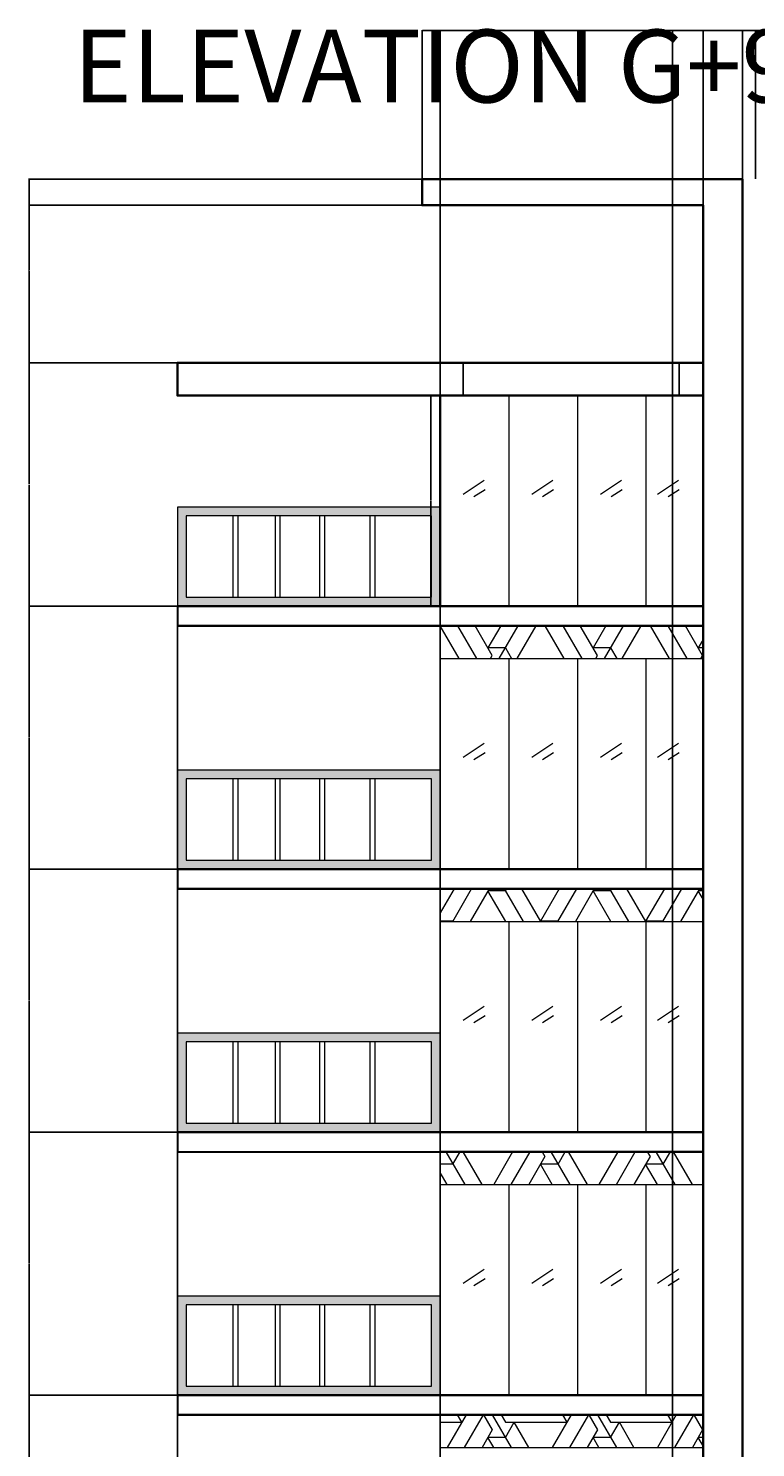
# Model space of a CAD drawing. Units: inches. Extents: x -38 to 698, y -57 to 1364.
# Tile 4 of 5: x -38 to 294, y 716 to 1364. Entities that reach past the tile are written whole.
import ezdxf

# ---------------------------------------------------------------- set-up
doc = ezdxf.new("R2010")
doc.units = ezdxf.units.IN
doc.header["$MEASUREMENT"] = 0
for name, color, linetype, lineweight in [('A-ANNO-DIMS', 2, 'Continuous', 18), ('A-ANNO-TEXT', 7, 'Continuous', 25), ('A-ELEV-PATT', 8, 'Continuous', 13), ('A-FLOR', 7, 'Continuous', 30), ('A-FLOR-HRAL', 7, 'Continuous', 20), ('A-GLAZ', 4, 'Continuous', 18), ('A-ROOF', 7, 'Continuous', 35), ('A-WALL', 7, 'Continuous', 35), ('A-WALL-PATT', 8, 'Continuous', 13)]:
    doc.layers.add(name, color=color, linetype=linetype, lineweight=lineweight)
doc.styles.get("Standard").update_dxf_attribs({"font": 'arial.ttf'})
doc.dimstyles.get("Standard").update_dxf_attribs({"dimtxt": 0.18, "dimasz": 0.18, "dimexe": 0.18, "dimexo": 0.0625, "dimgap": 0.09, "dimtad": 0, "dimtih": 1, "dimtoh": 1, "dimdec": 4, "dimzin": 0, "dimdsep": 46, "dimtxsty": 'Standard', "dimcen": 0.09, "dimadec": 0, "dimazin": 0, "dimtfac": 1, "dimtdec": 4, "dimtofl": 0, "dimtmove": 0, "dimatfit": 3, "dimfxl": 1, "dimtolj": 1, "dimtzin": 0, "dimarcsym": 0})

# ---------------------------------------------------------------- blocks, each defined once
blk = doc.blocks.new('WINDOW-4L-LH')
for p, q in [((20.81, 96), (20.81, 0)), ((52.11, 96), (52.11, 0)), ((83.42, 96), (83.42, 0)), ((0, 50.99), (9.6, 57.46)), ((4.92, 50.03), (9.96, 53.14)), ((31.3, 50.99), (40.9, 57.46)), ((36.22, 50.03), (41.26, 53.14)), ((62.61, 50.99), (72.2, 57.46)), ((67.52, 50.03), (72.56, 53.14)), ((88.7, 50.99), (98.29, 57.46)), ((93.61, 50.03), (98.65, 53.14))]:
    blk.add_line(p, q)
blk = doc.blocks.new('BALCONY-GUARD-PICKETS')
for p, q in [((0, 37.13), (0, 0)), ((2.41, 0), (2.41, 37.13)), ((19.25, 37.13), (19.25, 0)), ((21.65, 0), (21.65, 37.13)), ((39.53, 37.13), (39.53, 0)), ((41.93, 0), (41.93, 37.13)), ((62.55, 37.13), (62.55, 0)), ((64.96, 0), (64.96, 37.13))]:
    blk.add_line(p, q)
blk = doc.blocks.new('*D10')
at = {"layer": 'A-ANNO-DIMS', "color": 0, "lineweight": -2, "transparency": 16777216}
for p, q in [((160.18, 1196.28), (160.18, 1211.19)), ((160.36, 1211.01), (208.2, 1211.01)), ((258.65, 1211.01), (210.81, 1211.01)), ((258.83, 1196.28), (258.83, 1211.19))]:
    blk.add_line(p, q, dxfattribs=at)
at = {"layer": 'A-ANNO-DIMS', "color": 0, "transparency": 16777216}
for points in [[(160.36, 1211.04), (160.36, 1210.98), (160.18, 1211.01)], [(258.65, 1211.04), (258.65, 1210.98), (258.83, 1211.01)]]:
    blk.add_solid(points, dxfattribs=at)
at = {"layer": 'Defpoints', "color": 0, "transparency": 16777216}
for p in [(258.83, 1211.01), (160.18, 1196.21), (258.83, 1196.21)]:
    blk.add_point(p, dxfattribs=at)
at = {"layer": 'A-ANNO-DIMS', "color": 0, "transparency": 16777216, "insert": (209.51, 1211.01), "char_height": 0.18, "attachment_point": 5}
blk.add_mtext('\\A1;LH WINDOW 99 TYP.', dxfattribs=at)
blk = doc.blocks.new('*D11')
at = {"layer": 'A-ANNO-DIMS', "color": 0, "lineweight": -2, "transparency": 16777216}
for p, q in [((160.12, 1196.21), (145.2, 1196.21)), ((145.38, 1196.03), (145.38, 1148.4)), ((145.38, 1100.39), (145.38, 1148.03)), ((160.12, 1100.21), (145.2, 1100.21))]:
    blk.add_line(p, q, dxfattribs=at)
at = {"layer": 'A-ANNO-DIMS', "color": 0, "transparency": 16777216}
for points in [[(145.35, 1196.03), (145.41, 1196.03), (145.38, 1196.21)], [(145.35, 1100.39), (145.41, 1100.39), (145.38, 1100.21)]]:
    blk.add_solid(points, dxfattribs=at)
at = {"layer": 'Defpoints', "color": 0, "transparency": 16777216}
for p in [(145.38, 1196.21), (160.18, 1196.21), (160.18, 1100.21)]:
    blk.add_point(p, dxfattribs=at)
at = {"layer": 'A-ANNO-DIMS', "color": 0, "transparency": 16777216, "insert": (145.38, 1148.21), "char_height": 0.18, "attachment_point": 5}
blk.add_mtext('\\A1;96 TYP.', dxfattribs=at)
blk = doc.blocks.new('*D24')
at = {"layer": 'A-ANNO-DIMS', "color": 0, "lineweight": -2, "transparency": 16777216}
for p, q in [((29.69, 1100.15), (29.69, -56.67)), ((269.69, 1100.15), (269.69, -56.67)), ((29.87, -56.49), (149.4, -56.49)), ((269.51, -56.49), (149.98, -56.49))]:
    blk.add_line(p, q, dxfattribs=at)
at = {"layer": 'A-ANNO-DIMS', "color": 0, "transparency": 16777216}
for points in [[(29.87, -56.46), (29.87, -56.52), (29.69, -56.49)], [(269.51, -56.46), (269.51, -56.52), (269.69, -56.49)]]:
    blk.add_solid(points, dxfattribs=at)
at = {"layer": 'Defpoints', "color": 0, "transparency": 16777216}
for p in [(29.69, 1100.21), (269.69, 1100.21), (269.69, -56.49)]:
    blk.add_point(p, dxfattribs=at)
at = {"layer": 'A-ANNO-DIMS', "color": 0, "transparency": 16777216, "insert": (149.69, -56.49), "char_height": 0.18, "attachment_point": 5}
blk.add_mtext('\\A1;240', dxfattribs=at)
blk = doc.blocks.new('*D25')
at = {"layer": 'A-ANNO-DIMS', "color": 0, "lineweight": -2, "transparency": 16777216}
for p, q in [((269.69, 1100.15), (269.69, -56.67)), ((389.69, 1100.15), (389.69, -56.67)), ((269.87, -56.49), (329.41, -56.49)), ((389.51, -56.49), (329.97, -56.49))]:
    blk.add_line(p, q, dxfattribs=at)
at = {"layer": 'A-ANNO-DIMS', "color": 0, "transparency": 16777216}
for points in [[(269.87, -56.46), (269.87, -56.52), (269.69, -56.49)], [(389.51, -56.46), (389.51, -56.52), (389.69, -56.49)]]:
    blk.add_solid(points, dxfattribs=at)
at = {"layer": 'Defpoints', "color": 0, "transparency": 16777216}
for p in [(269.69, 1100.21), (389.69, 1100.21), (389.69, -56.49)]:
    blk.add_point(p, dxfattribs=at)
at = {"layer": 'A-ANNO-DIMS', "color": 0, "transparency": 16777216, "insert": (329.69, -56.49), "char_height": 0.18, "attachment_point": 5}
blk.add_mtext('\\A1;120', dxfattribs=at)
blk = doc.blocks.new('*D27')
at = {"layer": 'A-ANNO-DIMS', "color": 0, "lineweight": -2, "transparency": 16777216}
for p, q in [((149.69, 380.28), (149.69, 1362.92)), ((149.87, 1362.74), (209.41, 1362.74)), ((269.51, 1362.74), (209.97, 1362.74)), ((269.69, 380.28), (269.69, 1362.92))]:
    blk.add_line(p, q, dxfattribs=at)
at = {"layer": 'A-ANNO-DIMS', "color": 0, "transparency": 16777216}
for points in [[(149.87, 1362.77), (149.87, 1362.71), (149.69, 1362.74)], [(269.51, 1362.77), (269.51, 1362.71), (269.69, 1362.74)]]:
    blk.add_solid(points, dxfattribs=at)
at = {"layer": 'Defpoints', "color": 0, "transparency": 16777216}
for p in [(269.69, 1362.74), (149.69, 380.21), (269.69, 380.21)]:
    blk.add_point(p, dxfattribs=at)
at = {"layer": 'A-ANNO-DIMS', "color": 0, "transparency": 16777216, "insert": (209.69, 1362.74), "char_height": 0.18, "attachment_point": 5}
blk.add_mtext('\\A1;120', dxfattribs=at)
blk = doc.blocks.new('*D34')
at = {"layer": 'A-ANNO-DIMS', "color": 0, "lineweight": -2, "transparency": 16777216}
for p, q in [((29.62, 740.21), (-38.19, 740.21)), ((-38.01, 740.03), (-38.01, 680.4)), ((-38.01, 620.39), (-38.01, 680.03)), ((29.62, 620.21), (-38.19, 620.21))]:
    blk.add_line(p, q, dxfattribs=at)
at = {"layer": 'A-ANNO-DIMS', "color": 0, "transparency": 16777216}
for points in [[(-38.04, 740.03), (-37.98, 740.03), (-38.01, 740.21)], [(-38.04, 620.39), (-37.98, 620.39), (-38.01, 620.21)]]:
    blk.add_solid(points, dxfattribs=at)
at = {"layer": 'Defpoints', "color": 0, "transparency": 16777216}
for p in [(-38.01, 740.21), (29.69, 740.21), (29.69, 620.21)]:
    blk.add_point(p, dxfattribs=at)
at = {"layer": 'A-ANNO-DIMS', "color": 0, "transparency": 16777216, "insert": (-38.01, 680.21), "char_height": 0.18, "attachment_point": 5}
blk.add_mtext('\\A1;120', dxfattribs=at)
blk = doc.blocks.new('*D35')
at = {"layer": 'A-ANNO-DIMS', "color": 0, "lineweight": -2, "transparency": 16777216}
for p, q in [((29.62, 860.21), (-38.19, 860.21)), ((-38.01, 860.03), (-38.01, 800.4)), ((-38.01, 740.39), (-38.01, 800.03)), ((29.62, 740.21), (-38.19, 740.21))]:
    blk.add_line(p, q, dxfattribs=at)
at = {"layer": 'A-ANNO-DIMS', "color": 0, "transparency": 16777216}
for points in [[(-38.04, 860.03), (-37.98, 860.03), (-38.01, 860.21)], [(-38.04, 740.39), (-37.98, 740.39), (-38.01, 740.21)]]:
    blk.add_solid(points, dxfattribs=at)
at = {"layer": 'Defpoints', "color": 0, "transparency": 16777216}
for p in [(-38.01, 860.21), (29.69, 860.21), (29.69, 740.21)]:
    blk.add_point(p, dxfattribs=at)
at = {"layer": 'A-ANNO-DIMS', "color": 0, "transparency": 16777216, "insert": (-38.01, 800.21), "char_height": 0.18, "attachment_point": 5}
blk.add_mtext('\\A1;120', dxfattribs=at)
blk = doc.blocks.new('*D36')
at = {"layer": 'A-ANNO-DIMS', "color": 0, "lineweight": -2, "transparency": 16777216}
for p, q in [((29.62, 980.21), (-38.19, 980.21)), ((-38.01, 980.03), (-38.01, 920.4)), ((-38.01, 860.39), (-38.01, 920.03)), ((29.62, 860.21), (-38.19, 860.21))]:
    blk.add_line(p, q, dxfattribs=at)
at = {"layer": 'A-ANNO-DIMS', "color": 0, "transparency": 16777216}
for points in [[(-38.04, 980.03), (-37.98, 980.03), (-38.01, 980.21)], [(-38.04, 860.39), (-37.98, 860.39), (-38.01, 860.21)]]:
    blk.add_solid(points, dxfattribs=at)
at = {"layer": 'Defpoints', "color": 0, "transparency": 16777216}
for p in [(-38.01, 980.21), (29.69, 980.21), (29.69, 860.21)]:
    blk.add_point(p, dxfattribs=at)
at = {"layer": 'A-ANNO-DIMS', "color": 0, "transparency": 16777216, "insert": (-38.01, 920.21), "char_height": 0.18, "attachment_point": 5}
blk.add_mtext('\\A1;120', dxfattribs=at)
blk = doc.blocks.new('*D37')
at = {"layer": 'A-ANNO-DIMS', "color": 0, "lineweight": -2, "transparency": 16777216}
for p, q in [((29.62, 1100.21), (-38.19, 1100.21)), ((-38.01, 1100.03), (-38.01, 1040.4)), ((-38.01, 980.39), (-38.01, 1040.03)), ((29.62, 980.21), (-38.19, 980.21))]:
    blk.add_line(p, q, dxfattribs=at)
at = {"layer": 'A-ANNO-DIMS', "color": 0, "transparency": 16777216}
for points in [[(-38.04, 1100.03), (-37.98, 1100.03), (-38.01, 1100.21)], [(-38.04, 980.39), (-37.98, 980.39), (-38.01, 980.21)]]:
    blk.add_solid(points, dxfattribs=at)
at = {"layer": 'Defpoints', "color": 0, "transparency": 16777216}
for p in [(-38.01, 1100.21), (29.69, 1100.21), (29.69, 980.21)]:
    blk.add_point(p, dxfattribs=at)
at = {"layer": 'A-ANNO-DIMS', "color": 0, "transparency": 16777216, "insert": (-38.01, 1040.21), "char_height": 0.18, "attachment_point": 5}
blk.add_mtext('\\A1;120', dxfattribs=at)
blk = doc.blocks.new('*D38')
at = {"layer": 'A-ANNO-DIMS', "color": 0, "lineweight": -2, "transparency": 16777216}
for p, q in [((29.62, 1211.21), (-38.19, 1211.21)), ((-38.01, 1211.03), (-38.01, 1155.9)), ((-38.01, 1100.39), (-38.01, 1155.53)), ((29.62, 1100.21), (-38.19, 1100.21))]:
    blk.add_line(p, q, dxfattribs=at)
at = {"layer": 'A-ANNO-DIMS', "color": 0, "transparency": 16777216}
for points in [[(-38.04, 1211.03), (-37.98, 1211.03), (-38.01, 1211.21)], [(-38.04, 1100.39), (-37.98, 1100.39), (-38.01, 1100.21)]]:
    blk.add_solid(points, dxfattribs=at)
at = {"layer": 'Defpoints', "color": 0, "transparency": 16777216}
for p in [(-38.01, 1211.21), (29.69, 1211.21), (29.69, 1100.21)]:
    blk.add_point(p, dxfattribs=at)
at = {"layer": 'A-ANNO-DIMS', "color": 0, "transparency": 16777216, "insert": (-38.01, 1155.71), "char_height": 0.18, "attachment_point": 5}
blk.add_mtext('\\A1;111', dxfattribs=at)
blk = doc.blocks.new('*D39')
at = {"layer": 'A-ANNO-DIMS', "color": 0, "lineweight": -2, "transparency": 16777216}
for p, q in [((141.33, 1295.04), (-38.19, 1295.04)), ((-38.01, 1294.86), (-38.01, 1253.31)), ((-38.01, 1211.39), (-38.01, 1252.94)), ((29.62, 1211.21), (-38.19, 1211.21))]:
    blk.add_line(p, q, dxfattribs=at)
at = {"layer": 'A-ANNO-DIMS', "color": 0, "transparency": 16777216}
for points in [[(-38.04, 1294.86), (-37.98, 1294.86), (-38.01, 1295.04)], [(-38.04, 1211.39), (-37.98, 1211.39), (-38.01, 1211.21)]]:
    blk.add_solid(points, dxfattribs=at)
at = {"layer": 'Defpoints', "color": 0, "transparency": 16777216}
for p in [(-38.01, 1295.04), (141.39, 1295.04), (29.69, 1211.21)]:
    blk.add_point(p, dxfattribs=at)
at = {"layer": 'A-ANNO-DIMS', "color": 0, "transparency": 16777216, "insert": (-38.01, 1253.13), "char_height": 0.18, "attachment_point": 5}
blk.add_mtext('\\A1;83.82', dxfattribs=at)
blk = doc.blocks.new('*D43')
at = {"layer": 'A-ANNO-DIMS', "color": 0, "lineweight": -2, "transparency": 16777216}
for p, q in [((141.39, 1295.1), (141.39, 1362.92)), ((141.57, 1362.74), (214.15, 1362.74)), ((287.51, 1362.74), (214.92, 1362.74)), ((287.69, 1295.1), (287.69, 1362.92))]:
    blk.add_line(p, q, dxfattribs=at)
at = {"layer": 'A-ANNO-DIMS', "color": 0, "transparency": 16777216}
for points in [[(141.57, 1362.77), (141.57, 1362.71), (141.39, 1362.74)], [(287.51, 1362.77), (287.51, 1362.71), (287.69, 1362.74)]]:
    blk.add_solid(points, dxfattribs=at)
at = {"layer": 'Defpoints', "color": 0, "transparency": 16777216}
for p in [(287.69, 1362.74), (141.39, 1295.04), (287.69, 1295.04)]:
    blk.add_point(p, dxfattribs=at)
at = {"layer": 'A-ANNO-DIMS', "color": 0, "transparency": 16777216, "insert": (214.54, 1362.74), "char_height": 0.18, "attachment_point": 5}
blk.add_mtext('\\A1;146.3', dxfattribs=at)
blk = doc.blocks.new('*D45')
at = {"layer": 'A-ANNO-DIMS', "color": 0, "lineweight": -2, "transparency": 16777216}
for p, q in [((141.33, 1295.04), (-38.19, 1295.04)), ((-38.01, 1294.86), (-38.01, 1289.22)), ((-38.01, 1283.22), (-38.01, 1288.85)), ((141.33, 1283.04), (-38.19, 1283.04))]:
    blk.add_line(p, q, dxfattribs=at)
at = {"layer": 'A-ANNO-DIMS', "color": 0, "transparency": 16777216}
for points in [[(-38.04, 1294.86), (-37.98, 1294.86), (-38.01, 1295.04)], [(-38.04, 1283.22), (-37.98, 1283.22), (-38.01, 1283.04)]]:
    blk.add_solid(points, dxfattribs=at)
at = {"layer": 'Defpoints', "color": 0, "transparency": 16777216}
for p in [(-38.01, 1295.04), (141.39, 1295.04), (141.39, 1283.04)]:
    blk.add_point(p, dxfattribs=at)
at = {"layer": 'A-ANNO-DIMS', "color": 0, "transparency": 16777216, "insert": (-38.01, 1289.04), "char_height": 0.18, "attachment_point": 5}
blk.add_mtext('\\A1;12', dxfattribs=at)
blk = doc.blocks.new('*D48')
at = {"layer": 'A-ANNO-DIMS', "color": 0, "lineweight": -2, "transparency": 16777216}
for p, q in [((255.72, 101.28), (255.72, 1362.92)), ((255.9, 1362.74), (328.99, 1362.74)), ((402.85, 1362.74), (329.76, 1362.74)), ((403.03, 101.28), (403.03, 1362.92))]:
    blk.add_line(p, q, dxfattribs=at)
at = {"layer": 'A-ANNO-DIMS', "color": 0, "transparency": 16777216}
for points in [[(255.9, 1362.77), (255.9, 1362.71), (255.72, 1362.74)], [(402.85, 1362.77), (402.85, 1362.71), (403.03, 1362.74)]]:
    blk.add_solid(points, dxfattribs=at)
at = {"layer": 'Defpoints', "color": 0, "transparency": 16777216}
for p in [(403.03, 1362.74), (255.72, 101.21), (403.03, 101.21)]:
    blk.add_point(p, dxfattribs=at)
at = {"layer": 'A-ANNO-DIMS', "color": 0, "transparency": 16777216, "insert": (329.37, 1362.74), "char_height": 0.18, "attachment_point": 5}
blk.add_mtext('\\A1;147.3', dxfattribs=at)
blk = doc.blocks.new('*D52')
at = {"layer": 'A-ANNO-DIMS', "color": 0, "lineweight": -2, "transparency": 16777216}
for p, q in [((287.69, 1294.97), (287.69, -56.67)), ((269.69, 1282.97), (269.69, -56.67)), ((269.87, -56.49), (278.47, -56.49)), ((287.51, -56.49), (278.9, -56.49))]:
    blk.add_line(p, q, dxfattribs=at)
at = {"layer": 'A-ANNO-DIMS', "color": 0, "transparency": 16777216}
for points in [[(269.87, -56.46), (269.87, -56.52), (269.69, -56.49)], [(287.51, -56.46), (287.51, -56.52), (287.69, -56.49)]]:
    blk.add_solid(points, dxfattribs=at)
at = {"layer": 'Defpoints', "color": 0, "transparency": 16777216}
for p in [(287.69, 1295.04), (269.69, 1283.04), (287.69, -56.49)]:
    blk.add_point(p, dxfattribs=at)
at = {"layer": 'A-ANNO-DIMS', "color": 0, "transparency": 16777216, "insert": (278.69, -56.49), "char_height": 0.18, "attachment_point": 5}
blk.add_mtext('\\A1;18', dxfattribs=at)
blk = doc.blocks.new('*D53')
at = {"layer": 'A-ANNO-DIMS', "color": 0, "lineweight": -2, "transparency": 16777216}
for p, q in [((287.69, 1295.1), (287.69, 1362.92)), ((287.87, 1362.74), (290.54, 1362.74)), ((293.51, 1362.74), (290.83, 1362.74)), ((293.69, 1295.1), (293.69, 1362.92))]:
    blk.add_line(p, q, dxfattribs=at)
at = {"layer": 'A-ANNO-DIMS', "color": 0, "transparency": 16777216}
for points in [[(287.87, 1362.77), (287.87, 1362.71), (287.69, 1362.74)], [(293.51, 1362.77), (293.51, 1362.71), (293.69, 1362.74)]]:
    blk.add_solid(points, dxfattribs=at)
at = {"layer": 'Defpoints', "color": 0, "transparency": 16777216}
for p in [(293.69, 1362.74), (287.69, 1295.04), (293.69, 1295.04)]:
    blk.add_point(p, dxfattribs=at)
at = {"layer": 'A-ANNO-DIMS', "color": 0, "transparency": 16777216, "insert": (290.69, 1362.74), "char_height": 0.18, "attachment_point": 5}
blk.add_mtext('\\A1;6', dxfattribs=at)

msp = doc.modelspace()

# ---------------------------------------------------------------- hatches: boundary and pattern name
at = {"layer": 'A-ELEV-PATT', "transparency": 33554562}
h = msp.add_hatch(dxfattribs=at)
h.set_pattern_fill('HONEY', color=256, scale=40)
h.set_pattern_definition([(0, (-116.5534, -96.733), (7.5, 4.330127), [5, -10]), (120, (-116.5534, -96.733), (-7.5, 4.330127), [5, -10]), (60, (-116.5534, -96.733), (2e-15, 8.660254), [-10, 5])])
h.paths.add_polyline_path([(629.0638, 1145.3406), (509.0638, 1145.3406), (509.0638, 1100.2149), (629.0638, 1100.2149)])
h.paths.add_polyline_path([(625.0638, 1141.3406), (625.0638, 1104.2149), (513.0638, 1104.2149), (513.0638, 1141.3406)], flags=16)
h.paths.add_polyline_path([(629.0638, 1025.3406), (509.0638, 1025.3406), (509.0638, 980.2149), (629.0638, 980.2149)])
h.paths.add_polyline_path([(625.0638, 1021.3406), (625.0638, 984.2149), (513.0638, 984.2149), (513.0638, 1021.3406)], flags=16)
h.paths.add_polyline_path([(629.0638, 905.3406), (509.0638, 905.3406), (509.0638, 860.2149), (629.0638, 860.2149)])
h.paths.add_polyline_path([(625.0638, 901.3406), (625.0638, 864.2149), (513.0638, 864.2149), (513.0638, 901.3406)], flags=16)
h.paths.add_polyline_path([(629.0638, 785.3406), (509.0638, 785.3406), (509.0638, 740.2149), (629.0638, 740.2149)])
h.paths.add_polyline_path([(625.0638, 781.3406), (625.0638, 744.2149), (513.0638, 744.2149), (513.0638, 781.3406)], flags=16)
h.paths.add_polyline_path([(629.0638, 665.3406), (509.0638, 665.3406), (509.0638, 620.2149), (629.0638, 620.2149)])
h.paths.add_polyline_path([(625.0638, 661.3406), (625.0638, 624.2149), (513.0638, 624.2149), (513.0638, 661.3406)], flags=16)
h.paths.add_polyline_path([(629.0638, 545.3406), (509.0638, 545.3406), (509.0638, 500.2149), (629.0638, 500.2149)])
h.paths.add_polyline_path([(625.0638, 541.3406), (625.0638, 504.2149), (513.0638, 504.2149), (513.0638, 541.3406)], flags=16)
h.paths.add_polyline_path([(629.0638, 425.3406), (509.0638, 425.3406), (509.0638, 380.2149), (629.0638, 380.2149)])
h.paths.add_polyline_path([(625.0638, 421.3406), (625.0638, 384.2149), (513.0638, 384.2149), (513.0638, 421.3406)], flags=16)
h.paths.add_polyline_path([(629.0638, 296.3406), (509.0638, 296.3406), (509.0638, 251.2149), (629.0638, 251.2149)])
h.paths.add_polyline_path([(625.0638, 292.3406), (625.0638, 255.2149), (513.0638, 255.2149), (513.0638, 292.3406)], flags=16)
h.paths.add_polyline_path([(149.6854, 296.3406), (29.6854, 296.3406), (29.6854, 251.2149), (149.6854, 251.2149)])
h.paths.add_polyline_path([(145.6854, 292.3406), (145.6854, 255.2149), (33.6854, 255.2149), (33.6854, 292.3406)], flags=16)
h.paths.add_polyline_path([(149.6854, 425.3406), (29.6854, 425.3406), (29.6854, 380.2149), (149.6854, 380.2149)])
h.paths.add_polyline_path([(145.6854, 421.3406), (145.6854, 384.2149), (33.6854, 384.2149), (33.6854, 421.3406)], flags=16)
h.paths.add_polyline_path([(149.6854, 545.3406), (29.6854, 545.3406), (29.6854, 500.2149), (149.6854, 500.2149)])
h.paths.add_polyline_path([(33.6854, 504.2149), (33.6854, 541.3406), (145.6854, 541.3406), (145.6854, 504.2149)], flags=16)
h.paths.add_polyline_path([(149.6854, 665.3406), (29.6854, 665.3406), (29.6854, 620.2149), (149.6854, 620.2149)])
h.paths.add_polyline_path([(33.6854, 624.2149), (33.6854, 661.3406), (145.6854, 661.3406), (145.6854, 624.2149)], flags=16)
h.paths.add_polyline_path([(149.6854, 785.3406), (29.6854, 785.3406), (29.6854, 740.2149), (149.6854, 740.2149)])
h.paths.add_polyline_path([(33.6854, 744.2149), (33.6854, 781.3406), (145.6854, 781.3406), (145.6854, 744.2149)], flags=16)
h.paths.add_polyline_path([(149.6854, 905.3406), (29.6854, 905.3406), (29.6854, 860.2149), (149.6854, 860.2149)])
h.paths.add_polyline_path([(145.6854, 901.3406), (145.6854, 864.2149), (33.6854, 864.2149), (33.6854, 901.3406)], flags=16)
h.paths.add_polyline_path([(149.6854, 1025.3406), (29.6854, 1025.3406), (29.6854, 980.2149), (149.6854, 980.2149)])
h.paths.add_polyline_path([(33.6854, 984.2149), (33.6854, 1021.3406), (145.6854, 1021.3406), (145.6854, 984.2149)], flags=16)
h.paths.add_polyline_path([(149.6854, 1145.3406), (29.6854, 1145.3406), (29.6854, 1100.2149), (149.6854, 1100.2149)])
h.paths.add_polyline_path([(33.6854, 1104.2149), (33.6854, 1141.3406), (145.6854, 1141.3406), (145.6854, 1104.2149)], flags=16)
at = {"layer": 'A-WALL-PATT', "transparency": 33554562}
h = msp.add_hatch(dxfattribs=at)
h.set_pattern_fill('ESCHER', color=256, scale=40)
h.set_pattern_definition([(60, (-116.553, -96.733), (-48, -1e-08), [44, -4]), (180, (-116.553, -96.733), (24, -41.5692), [44, -4]), (300, (-116.553, -96.733), (48, -1e-08), [44, -4]), (60, (-112.553, -96.733), (-48, -1e-08), [8, -40]), (300, (-112.553, -96.733), (48, -1e-08), [8, -40]), (60, (-118.553, -93.27), (-48, -1e-08), [8, -40]), (180, (-118.553, -93.27), (24, -41.5692), [8, -40]), (300, (-118.553, -100.197), (48, -1e-08), [8, -40]), (180, (-118.553, -100.197), (24, -41.5692), [8, -40]), (60, (-132.553, -96.733), (-48, -1e-08), [8, -40]), (300, (-132.553, -96.733), (48, -1e-08), [8, -40]), (60, (-108.553, -110.59), (-48, -1e-08), [8, -40]), (180, (-108.553, -110.59), (24, -41.5692), [8, -40]), (300, (-108.553, -82.877), (48, -1e-08), [8, -40]), (180, (-108.553, -82.877), (24, -41.5692), [8, -40]), (0, (-108.553, -89.805), (-24, 41.5692), [28, -20]), (0, (-108.553, -103.66), (-24, 41.5692), [28, -20]), (120, (-114.553, -86.34), (-48, 1e-08), [28, -20]), (120, (-126.553, -93.27), (-48, 1e-08), [28, -20]), (240, (-126.553, -100.197), (24, -41.5692), [28, -20]), (240, (-114.553, -107.125), (24, -41.5692), [28, -20])])
h.paths.add_polyline_path([(269.6854, 371.2149), (149.6854, 371.2149), (149.6854, 347.2149), (269.6854, 347.2149)])
h.paths.add_polyline_path([(509.0638, 371.2149), (389.6854, 371.2149), (389.6854, 347.2149), (509.0638, 347.2149)])
h.paths.add_polyline_path([(269.6854, 491.2149), (149.6854, 491.2149), (149.6854, 476.2149), (269.6854, 476.2149)])
h.paths.add_polyline_path([(509.0638, 491.2149), (389.6854, 491.2149), (389.6854, 476.2149), (509.0638, 476.2149)])
h.paths.add_polyline_path([(509.0638, 611.2149), (389.6854, 611.2149), (389.6854, 596.2149), (509.0638, 596.2149)])
h.paths.add_polyline_path([(269.6854, 611.2149), (149.6854, 611.2149), (149.6854, 596.2149), (269.6854, 596.2149)])
h.paths.add_polyline_path([(269.6854, 731.2149), (149.6854, 731.2149), (149.6854, 716.2149), (269.6854, 716.2149)])
h.paths.add_polyline_path([(509.0638, 731.2149), (389.6854, 731.2149), (389.6854, 716.2149), (509.0638, 716.2149)])
h.paths.add_polyline_path([(509.0638, 851.2149), (389.6854, 851.2149), (389.6854, 836.2149), (509.0638, 836.2149)])
h.paths.add_polyline_path([(269.6854, 851.2149), (149.6854, 851.2149), (149.6854, 836.2149), (269.6854, 836.2149)])
h.paths.add_polyline_path([(269.6854, 971.2149), (149.6854, 971.2149), (149.6854, 956.2149), (269.6854, 956.2149)])
h.paths.add_polyline_path([(509.0638, 971.2149), (389.6854, 971.2149), (389.6854, 956.2149), (509.0638, 956.2149)])
h.paths.add_polyline_path([(509.0638, 1091.2149), (389.6854, 1091.2149), (389.6854, 1076.2149), (509.0638, 1076.2149)])
h.paths.add_polyline_path([(269.6854, 1091.2149), (149.6854, 1091.2149), (149.6854, 1076.2149), (269.6854, 1076.2149)])

# ---------------------------------------------------------------- linework, layer by layer
at = {"layer": 'A-FLOR'}
for points in [[(29.6854, 1100.2149), (269.6854, 1100.2149), (29.6854, 1100.2149), (29.6854, 1091.2149), (269.6854, 1091.2149), (29.6854, 1091.2149)], [(29.6854, 980.2149), (269.6854, 980.2149), (29.6854, 980.2149), (29.6854, 971.2149), (269.6854, 971.2149), (29.6854, 971.2149)], [(29.6854, 860.2149), (269.6854, 860.2149), (29.6854, 860.2149), (29.6854, 851.2149), (269.6854, 851.2149), (149.6854, 851.2149)], [(29.6854, 740.2149), (269.6854, 740.2149), (29.6854, 740.2149), (29.6854, 731.2149), (269.6854, 731.2149), (29.6854, 731.2149)]]:
    msp.add_lwpolyline(points, dxfattribs=at)
at = {"layer": 'A-FLOR-HRAL'}
for points in [[(149.6854, 1145.3406), (29.6854, 1145.3406), (29.6854, 1100.2149), (149.6854, 1100.2149)], [(145.6854, 1141.3406), (33.6854, 1141.3406), (33.6854, 1104.2149), (145.6854, 1104.2149)], [(149.6854, 1025.3406), (29.6854, 1025.3406), (29.6854, 980.2149), (149.6854, 980.2149)], [(145.6854, 1021.3406), (33.6854, 1021.3406), (33.6854, 984.2149), (145.6854, 984.2149)], [(149.6854, 905.3406), (29.6854, 905.3406), (29.6854, 860.2149), (149.6854, 860.2149)], [(145.6854, 901.3406), (33.6854, 901.3406), (33.6854, 864.2149), (145.6854, 864.2149)], [(149.6854, 785.3406), (29.6854, 785.3406), (29.6854, 740.2149), (149.6854, 740.2149)], [(145.6854, 781.3406), (33.6854, 781.3406), (33.6854, 744.2149), (145.6854, 744.2149)]]:
    msp.add_lwpolyline(points, close=True, dxfattribs=at)
at = {"layer": 'A-GLAZ'}
for p, q in [((149.6854, 1076.2149), (269.6854, 1076.2149)), ((149.6854, 956.2149), (269.6854, 956.2149)), ((149.6854, 836.2149), (269.6854, 836.2149)), ((149.6854, 716.2149), (269.6854, 716.2149))]:
    msp.add_line(p, q, dxfattribs=at)
for points in [[(149.6854, 980.2149), (149.6854, 1091.2149)], [(149.6854, 860.2149), (149.6854, 971.2149)], [(149.6854, 740.2149), (149.6854, 851.2149)], [(149.6854, 620.2149), (149.6854, 731.2149)]]:
    msp.add_lwpolyline(points, close=True, dxfattribs=at)
at = {"layer": 'A-ROOF'}
msp.add_lwpolyline([(269.6854, 1196.2149), (149.6854, 1196.2149), (149.6854, 1100.2149), (149.6854, 1196.2149), (29.6854, 1196.2149), (29.6854, 1211.2149), (269.6854, 1211.2149), (141.3895, 1211.2149)], dxfattribs=at)
at = {"layer": 'A-WALL'}
msp.add_lwpolyline([(269.6854, 107.2149), (269.6854, 851.2149), (269.6854, 971.2149), (269.6854, 1283.0353), (141.3895, 1283.0353), (141.3895, 1295.0353), (287.6854, 1295.0353), (287.6854, 971.2149), (287.6854, 851.2149), (287.6854, 107.2149)], dxfattribs=at)

# ---------------------------------------------------------------- block references
at = {"layer": 'A-FLOR-HRAL'}
for p in [(55.02, 1104.215), (55.02, 984.215), (55.02, 864.215), (55.02, 744.215)]:
    msp.add_blockref('BALCONY-GUARD-PICKETS', p, dxfattribs=at)
at = {"layer": 'A-GLAZ'}
for p in [(160.18, 1100.215), (160.18, 980.215), (160.18, 860.215), (160.18, 740.215)]:
    msp.add_blockref('WINDOW-4L-LH', p, dxfattribs=at)

# ---------------------------------------------------------------- texts
at = {"layer": 'A-ANNO-TEXT'}
msp.add_text('ELEVATION G+9 ELEGENT DESIGN', height=33.216729, dxfattribs=at).set_placement((-17.7381, 1329.9565))

# ---------------------------------------------------------------- dimensions: what is measured, and where the dimension line sits
at = {"layer": 'A-ANNO-DIMS'}
for base, p1, p2, override, picture, middle in [((287.6854, 1362.7353), (141.3895, 1295.0353), (287.6854, 1295.0353), {"dimdec": 1, "dimlfac": 1, "dimrnd": 0, "dimzin": 0, "dimdsep": 46, "dimlunit": 2}, '*D43', (214.5375, 1362.7353)), ((269.6854, 1362.7353), (149.6854, 380.2149), (269.6854, 380.2149), {"dimdec": 0, "dimlfac": 1, "dimrnd": 0, "dimzin": 0, "dimdsep": 46, "dimlunit": 2}, '*D27', (209.6854, 1362.7353)), ((403.029, 1362.7353), (255.7202, 101.2149), (403.029, 101.2149), {"dimdec": 1, "dimlfac": 1, "dimrnd": 0, "dimzin": 0, "dimdsep": 46, "dimlunit": 2}, '*D48', (329.3746, 1362.7353)), ((293.6854, 1362.7353), (287.6854, 1295.0353), (293.6854, 1295.0353), {"dimdec": 0, "dimlfac": 1, "dimrnd": 0, "dimzin": 0, "dimdsep": 46, "dimlunit": 2}, '*D53', (290.6854, 1362.7353)), ((287.6854, -56.4851), (269.6854, 1283.0353), (287.6854, 1295.0353), {"dimdec": 0, "dimlfac": 1, "dimrnd": 0, "dimzin": 0, "dimdsep": 46, "dimlunit": 2}, '*D52', (278.6854, -56.4851)), ((269.6854, -56.4851), (29.6854, 1100.2149), (269.6854, 1100.2149), {"dimdec": 0, "dimlfac": 1, "dimrnd": 0, "dimzin": 0, "dimdsep": 46, "dimlunit": 2}, '*D24', (149.6854, -56.4851)), ((389.6854, -56.4851), (269.6854, 1100.2149), (389.6854, 1100.2149), {"dimdec": 0, "dimlfac": 1, "dimrnd": 0, "dimzin": 0, "dimdsep": 46, "dimlunit": 2}, '*D25', (329.6854, -56.4851))]:
    dim = msp.add_linear_dim(base=base, p1=p1, p2=p2, dimstyle='Standard', override=override, dxfattribs=at)
    dim.commit()
    dim.dimension.update_dxf_attribs({"geometry": picture, "text_midpoint": middle})
for base, p1, p2, override, picture, middle in [((-38.0146, 1295.0353), (29.6854, 1211.2149), (141.3895, 1295.0353), {"dimdec": 2, "dimlfac": 1, "dimrnd": 0, "dimzin": 0, "dimdsep": 46, "dimlunit": 2}, '*D39', (-38.0146, 1253.1251)), ((-38.0146, 1295.0353), (141.3895, 1283.0353), (141.3895, 1295.0353), {"dimdec": 0, "dimlfac": 1, "dimrnd": 0, "dimzin": 0, "dimdsep": 46, "dimlunit": 2}, '*D45', (-38.0146, 1289.0353)), ((-38.0146, 1211.2149), (29.6854, 1100.2149), (29.6854, 1211.2149), {"dimdec": 0, "dimlfac": 1, "dimrnd": 0, "dimzin": 0, "dimdsep": 46, "dimlunit": 2}, '*D38', (-38.0146, 1155.7149)), ((-38.0146, 1100.2149), (29.6854, 980.2149), (29.6854, 1100.2149), {"dimdec": 0, "dimlfac": 1, "dimrnd": 0, "dimzin": 0, "dimdsep": 46, "dimlunit": 2}, '*D37', (-38.0146, 1040.2149)), ((-38.0146, 980.2149), (29.6854, 860.2149), (29.6854, 980.2149), {"dimdec": 0, "dimlfac": 1, "dimrnd": 0, "dimzin": 0, "dimdsep": 46, "dimlunit": 2}, '*D36', (-38.0146, 920.2149)), ((-38.0146, 860.2149), (29.6854, 740.2149), (29.6854, 860.2149), {"dimdec": 0, "dimlfac": 1, "dimrnd": 0, "dimzin": 0, "dimdsep": 46, "dimlunit": 2}, '*D35', (-38.0146, 800.2149)), ((-38.0146, 740.2149), (29.6854, 620.2149), (29.6854, 740.2149), {"dimdec": 0, "dimlfac": 1, "dimrnd": 0, "dimzin": 0, "dimdsep": 46, "dimlunit": 2}, '*D34', (-38.0146, 680.2149))]:
    dim = msp.add_linear_dim(base=base, p1=p1, p2=p2, angle=90, dimstyle='Standard', override=override, dxfattribs=at)
    dim.commit()
    dim.dimension.update_dxf_attribs({"geometry": picture, "text_midpoint": middle})
dim = msp.add_linear_dim(base=(258.8334, 1211.013), p1=(160.1796, 1196.2149), p2=(258.8334, 1196.2149), text='LH WINDOW <> TYP.', dimstyle='Standard', override={"dimdec": 0, "dimlfac": 1, "dimrnd": 0, "dimzin": 0, "dimdsep": 46, "dimlunit": 2}, dxfattribs=at)
dim.commit()
dim.dimension.update_dxf_attribs({"geometry": '*D10', "text_midpoint": (209.5065, 1211.013)})
dim = msp.add_linear_dim(base=(145.3816, 1196.2149), p1=(160.1796, 1100.2149), p2=(160.1796, 1196.2149), angle=90, text='<> TYP.', dimstyle='Standard', override={"dimdec": 0, "dimlfac": 1, "dimrnd": 0, "dimzin": 0, "dimdsep": 46, "dimlunit": 2}, dxfattribs=at)
dim.commit()
dim.dimension.update_dxf_attribs({"geometry": '*D11', "text_midpoint": (145.3816, 1148.2149)})

doc.saveas('drawing.dxf')
